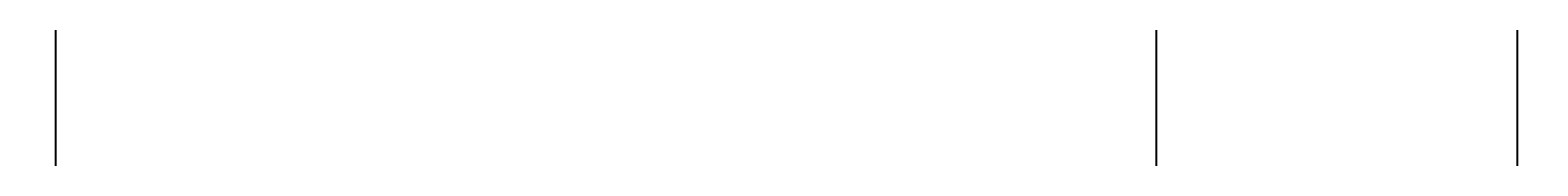
# Model space of a CAD drawing. Units: inches. Extents: x 35362 to 73946, y 43607 to 67532.
# Tile 78 of 134: x 50119 to 51337, y 47112 to 47206. Entities that reach past the tile are written whole.
import ezdxf

# ---------------------------------------------------------------- set-up
doc = ezdxf.new("R2010")
doc.units = ezdxf.units.IN
doc.header["$MEASUREMENT"] = 0
doc.layers.add('A-ANNO-DIMS', color=2, linetype='Continuous', lineweight=18)
doc.styles.get("Standard").update_dxf_attribs({"font": 'arial.ttf'})
doc.dimstyles.get("Standard").update_dxf_attribs({"dimtxt": 0.18, "dimasz": 0.18, "dimexe": 0.18, "dimexo": 0.0625, "dimgap": 0.09, "dimtad": 0, "dimtih": 1, "dimtoh": 1, "dimdec": 4, "dimzin": 0, "dimdsep": 46, "dimtxsty": 'Standard', "dimcen": 0.09, "dimadec": 0, "dimazin": 0, "dimtfac": 1, "dimtdec": 4, "dimtofl": 0, "dimtmove": 0, "dimatfit": 3, "dimfxl": 1, "dimtolj": 1, "dimtzin": 0, "dimarcsym": 0})

# ---------------------------------------------------------------- blocks, each defined once
blk = doc.blocks.new('*D11')
at = {"layer": 'A-ANNO-DIMS', "color": 0, "lineweight": -2, "transparency": 16777216}
for p, q in [((47978.7, 56028.8), (47978.7, 43606.7)), ((53109.8, 56028.8), (53109.8, 43606.7)), ((47978.8, 43606.9), (50543.9, 43606.9)), ((53109.6, 43606.9), (50544.6, 43606.9))]:
    blk.add_line(p, q, dxfattribs=at)
at = {"layer": 'A-ANNO-DIMS', "color": 0, "transparency": 16777216}
for points in [[(47978.8, 43606.9), (47978.8, 43606.8), (47978.7, 43606.9)], [(53109.6, 43606.9), (53109.6, 43606.8), (53109.8, 43606.9)]]:
    blk.add_solid(points, dxfattribs=at)
at = {"layer": 'Defpoints', "color": 0, "transparency": 16777216}
for p in [(47978.7, 56028.8), (53109.8, 56028.8), (53109.8, 43606.9)]:
    blk.add_point(p, dxfattribs=at)
at = {"layer": 'A-ANNO-DIMS', "color": 0, "transparency": 16777216, "insert": (50544.2, 43606.9), "char_height": 0.18, "attachment_point": 5}
blk.add_mtext('\\A1;5131', dxfattribs=at)
blk = doc.blocks.new('*D13')
at = {"layer": 'A-ANNO-DIMS', "color": 0, "lineweight": -2, "transparency": 16777216}
for p, q in [((48373.5, 51694), (48373.5, 43606.7)), ((51029, 51694), (51029, 43606.7)), ((48373.7, 43606.9), (49700.8, 43606.9)), ((51028.9, 43606.9), (49701.7, 43606.9))]:
    blk.add_line(p, q, dxfattribs=at)
at = {"layer": 'A-ANNO-DIMS', "color": 0, "transparency": 16777216}
for points in [[(48373.7, 43606.9), (48373.7, 43606.8), (48373.5, 43606.9)], [(51028.9, 43606.9), (51028.9, 43606.8), (51029, 43606.9)]]:
    blk.add_solid(points, dxfattribs=at)
at = {"layer": 'Defpoints', "color": 0, "transparency": 16777216}
for p in [(48373.5, 51694.1), (51029, 51694.1), (51029, 43606.9)]:
    blk.add_point(p, dxfattribs=at)
at = {"layer": 'A-ANNO-DIMS', "color": 0, "transparency": 16777216, "insert": (49701.3, 43606.9), "char_height": 0.18, "attachment_point": 5}
blk.add_mtext('\\A1;2655.6', dxfattribs=at)
blk = doc.blocks.new('*D17')
at = {"layer": 'A-ANNO-DIMS', "color": 0, "lineweight": -2, "transparency": 16777216}
for p, q in [((49923.3, 61293.2), (49923.3, 43606.7)), ((51913.9, 61293.2), (51913.9, 43606.7)), ((49923.5, 43606.9), (50918.2, 43606.9)), ((51913.8, 43606.9), (50919.1, 43606.9))]:
    blk.add_line(p, q, dxfattribs=at)
at = {"layer": 'A-ANNO-DIMS', "color": 0, "transparency": 16777216}
for points in [[(49923.5, 43606.9), (49923.5, 43606.8), (49923.3, 43606.9)], [(51913.8, 43606.9), (51913.8, 43606.8), (51913.9, 43606.9)]]:
    blk.add_solid(points, dxfattribs=at)
at = {"layer": 'Defpoints', "color": 0, "transparency": 16777216}
for p in [(49923.3, 61293.3), (51913.9, 61293.3), (51913.9, 43606.9)]:
    blk.add_point(p, dxfattribs=at)
at = {"layer": 'A-ANNO-DIMS', "color": 0, "transparency": 16777216, "insert": (50918.6, 43606.9), "char_height": 0.18, "attachment_point": 5}
blk.add_mtext('\\A1;1990.6', dxfattribs=at)
blk = doc.blocks.new('*D67')
at = {"layer": 'A-ANNO-DIMS', "color": 0, "lineweight": -2, "transparency": 16777216}
for p, q in [((56873.5, 53351.5), (35361.8, 53351.5)), ((35361.9, 53351.3), (35361.9, 49400.9)), ((35361.9, 45450.1), (35361.9, 49400.5)), ((53793.6, 45449.9), (35361.8, 45449.9))]:
    blk.add_line(p, q, dxfattribs=at)
at = {"layer": 'A-ANNO-DIMS', "color": 0, "transparency": 16777216}
for points in [[(35361.9, 53351.3), (35362, 53351.3), (35361.9, 53351.5)], [(35361.9, 45450.1), (35362, 45450.1), (35361.9, 45449.9)]]:
    blk.add_solid(points, dxfattribs=at)
at = {"layer": 'Defpoints', "color": 0, "transparency": 16777216}
for p in [(35361.9, 53351.5), (56873.6, 53351.5), (53793.6, 45449.9)]:
    blk.add_point(p, dxfattribs=at)
at = {"layer": 'A-ANNO-DIMS', "color": 0, "transparency": 16777216, "insert": (35361.9, 49400.7), "char_height": 0.18, "attachment_point": 5}
blk.add_mtext('\\A1;7901.6', dxfattribs=at)
blk = doc.blocks.new('*D90')
at = {"layer": 'A-ANNO-DIMS', "color": 0, "lineweight": -2, "transparency": 16777216}
for p, q in [((53707.7, 47291.3), (35361.8, 47291.3)), ((35361.9, 47291.1), (35361.9, 46710.3)), ((35361.9, 46129.1), (35361.9, 46709.9)), ((53793.6, 46128.9), (35361.8, 46128.9))]:
    blk.add_line(p, q, dxfattribs=at)
at = {"layer": 'A-ANNO-DIMS', "color": 0, "transparency": 16777216}
for points in [[(35361.9, 47291.1), (35362, 47291.1), (35361.9, 47291.3)], [(35361.9, 46129.1), (35362, 46129.1), (35361.9, 46128.9)]]:
    blk.add_solid(points, dxfattribs=at)
at = {"layer": 'Defpoints', "color": 0, "transparency": 16777216}
for p in [(53707.8, 47291.3), (35361.9, 46128.9), (53793.6, 46128.9)]:
    blk.add_point(p, dxfattribs=at)
at = {"layer": 'A-ANNO-DIMS', "color": 0, "transparency": 16777216, "insert": (35361.9, 46710.1), "char_height": 0.18, "attachment_point": 5}
blk.add_mtext('\\A1;1162.4', dxfattribs=at)
blk = doc.blocks.new('*D107')
at = {"layer": 'A-ANNO-DIMS', "color": 0, "lineweight": -2, "transparency": 16777216}
for p, q in [((50139.6, 59850), (50139.6, 43606.7)), ((51320.8, 59850), (51320.8, 43606.7)), ((50139.7, 43606.9), (50729.7, 43606.9)), ((51320.6, 43606.9), (50730.6, 43606.9))]:
    blk.add_line(p, q, dxfattribs=at)
at = {"layer": 'A-ANNO-DIMS', "color": 0, "transparency": 16777216}
for points in [[(50139.7, 43606.9), (50139.7, 43606.8), (50139.6, 43606.9)], [(51320.6, 43606.9), (51320.6, 43606.8), (51320.8, 43606.9)]]:
    blk.add_solid(points, dxfattribs=at)
at = {"layer": 'Defpoints', "color": 0, "transparency": 16777216}
for p in [(50139.6, 59850.1), (51320.8, 59850.1), (51320.8, 43606.9)]:
    blk.add_point(p, dxfattribs=at)
at = {"layer": 'A-ANNO-DIMS', "color": 0, "transparency": 16777216, "insert": (50730.2, 43606.9), "char_height": 0.18, "attachment_point": 5}
blk.add_mtext('\\A1;1181.3', dxfattribs=at)

msp = doc.modelspace()

# ---------------------------------------------------------------- dimensions: what is measured, and where the dimension line sits
at = {"layer": 'A-ANNO-DIMS'}
for base, p1, p2, override, picture, middle in [((51913.931, 43606.859), (49923.307, 61293.286), (51913.931, 61293.286), {"dimdec": 1, "dimlfac": 1, "dimrnd": 0, "dimzin": 0, "dimdsep": 46, "dimlunit": 2}, '*D17', (50918.619, 43606.859)), ((51320.8133, 43606.859), (50139.5627, 59850.0769), (51320.8133, 59850.0769), {"dimdec": 1, "dimlfac": 1, "dimrnd": 0, "dimzin": 0, "dimdsep": 46, "dimlunit": 2}, '*D107', (50730.188, 43606.859)), ((53109.76, 43606.859), (47978.665, 56028.836), (53109.76, 56028.836), {"dimdec": 0, "dimlfac": 1, "dimrnd": 0, "dimzin": 0, "dimdsep": 46, "dimlunit": 2}, '*D11', (50544.212, 43606.859)), ((51029.043, 43606.859), (48373.492, 51694.087), (51029.043, 51694.087), {"dimdec": 1, "dimlfac": 1, "dimrnd": 0, "dimzin": 0, "dimdsep": 46, "dimlunit": 2}, '*D13', (49701.267, 43606.859))]:
    dim = msp.add_linear_dim(base=base, p1=p1, p2=p2, dimstyle='Standard', override=override, dxfattribs=at)
    dim.commit()
    dim.dimension.update_dxf_attribs({"geometry": picture, "text_midpoint": middle})
for base, p1, p2, picture, middle in [((35361.949, 53351.529), (53793.638, 45449.894), (56873.602, 53351.529), '*D67', (35361.949, 49400.712)), ((35361.949, 46128.878), (53707.781, 47291.285), (53793.638, 46128.878), '*D90', (35361.949, 46710.081))]:
    dim = msp.add_linear_dim(base=base, p1=p1, p2=p2, angle=90, dimstyle='Standard', override={"dimdec": 1, "dimlfac": 1, "dimrnd": 0, "dimzin": 0, "dimdsep": 46, "dimlunit": 2}, dxfattribs=at)
    dim.commit()
    dim.dimension.update_dxf_attribs({"geometry": picture, "text_midpoint": middle})

doc.saveas('drawing.dxf')
